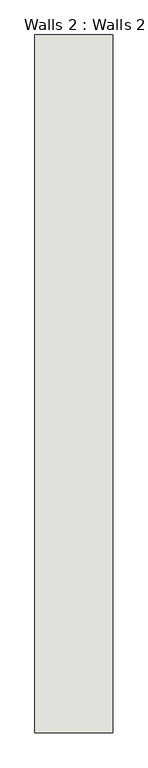
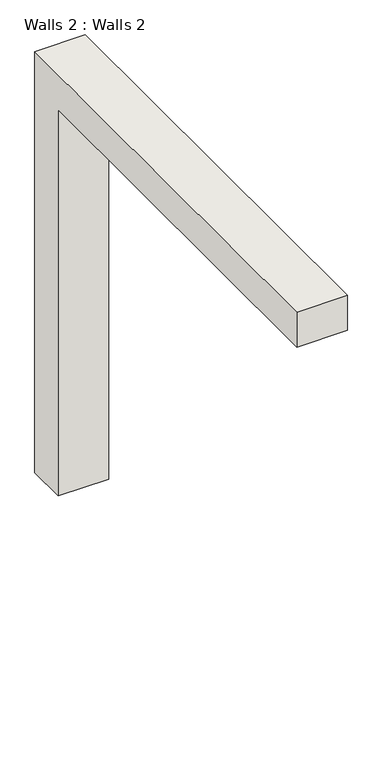
"""IFC4 building model written with IfcOpenShell, lengths in millimetres: wall geometry, Walls 2 : Walls 2."""

from ifc_helpers import new_model, si_unit, frame, origin, place, context, project, spatial, polyline, outline, extrude, source, transform, mapped, element, save


def walls_2_walls_2_c4a6eebc(model_context):
    return source(origin(), model_context, "Body", "SweptSolid", [
        extrude(outline(polyline([(9140.7756066, 11277.6), (9140.7756066, 7620.0), (8810.5756066, 7620.0), (8810.5756066, 10972.8), (5410.7832269, 10972.8), (5410.7832269, 11277.6), (9140.7756066, 11277.6)])), frame((-6980.0236868, 0.0, 0.0), z_axis=(1.0, 0.0, 0.0), x_axis=(0.0, 1.0, 0.0)), (0.0, 0.0, 1.0), 415.4741408),
    ])


if __name__ == "__main__":
    model = new_model("IFC4")
    model_context = context("Model", 3, world=origin())
    ifc_project = project(units=[si_unit("LENGTHUNIT", "METRE", prefix="MILLI")], contexts=[model_context])
    site = spatial("IfcSite", under=ifc_project)
    building = spatial("IfcBuilding", under=site)
    placement = place(None, origin())
    walls_2_walls_2_shape = walls_2_walls_2_c4a6eebc(model_context)
    element("IfcWall", 1, ObjectType="Walls 2 : Walls 2", at=placement, inside=building, context=model_context, shape_type="MappedRepresentation", body=[
        mapped(walls_2_walls_2_shape, transform((0.0, 0.0, 0.0), x_axis=(1.0, 0.0, 0.0), y_axis=(0.0, 1.0, 0.0), z_axis=(0.0, 0.0, 1.0))),
    ])
    save(model, "model.ifc")

# Revit data of these elements
# Element 1 (IfcWall, "Walls 2 : Walls 2")
#   Materials on its faces: "Default Wall"
# Materials
#   "Default Wall": colour RGB 128 128 128, transparency 0
